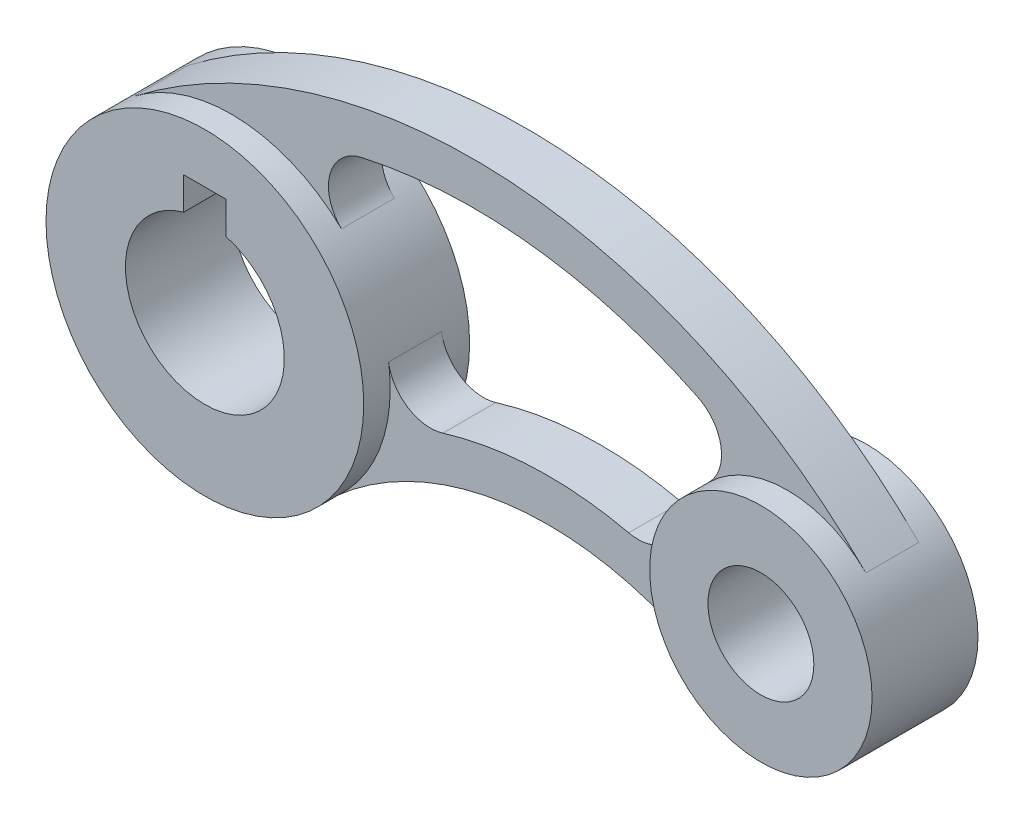
ISO-10303-21;
HEADER;
FILE_DESCRIPTION(('STEP AP214'),'2;1');
FILE_NAME('part.step','',(''),(''),'','','');
FILE_SCHEMA(('AUTOMOTIVE_DESIGN { 1 0 10303 214 1 1 1 1 }'));
ENDSEC;
DATA;
#1=APPLICATION_CONTEXT('core data for automotive mechanical design processes');
#2=APPLICATION_PROTOCOL_DEFINITION('international standard','automotive_design',2000,#1);
#3=PRODUCT_CONTEXT('',#1,'mechanical');
#4=PRODUCT('Part','Part','',(#3));
#5=PRODUCT_RELATED_PRODUCT_CATEGORY('part','',(#4));
#6=PRODUCT_DEFINITION_FORMATION('','',#4);
#7=PRODUCT_DEFINITION_CONTEXT('part definition',#1,'design');
#8=PRODUCT_DEFINITION('design','',#6,#7);
#9=PRODUCT_DEFINITION_SHAPE('','',#8);
#10=(LENGTH_UNIT() NAMED_UNIT(*) SI_UNIT(.MILLI.,.METRE.));
#11=(NAMED_UNIT(*) PLANE_ANGLE_UNIT() SI_UNIT($,.RADIAN.));
#12=(NAMED_UNIT(*) SI_UNIT($,.STERADIAN.) SOLID_ANGLE_UNIT());
#13=UNCERTAINTY_MEASURE_WITH_UNIT(LENGTH_MEASURE(1.E-05),#10,'distance_accuracy_value','');
#14=(GEOMETRIC_REPRESENTATION_CONTEXT(3) GLOBAL_UNCERTAINTY_ASSIGNED_CONTEXT((#13)) GLOBAL_UNIT_ASSIGNED_CONTEXT((#10,
#11,#12)) REPRESENTATION_CONTEXT('',''));
#15=CARTESIAN_POINT('',(0.,0.,0.));
#16=DIRECTION('',(0.,0.,1.));
#17=DIRECTION('',(1.,0.,0.));
#18=AXIS2_PLACEMENT_3D('',#15,#16,#17);
#19=CARTESIAN_POINT('',(-105.,0.,-10.));
#20=DIRECTION('',(0.,0.,1.));
#21=DIRECTION('',(1.,0.,0.));
#22=AXIS2_PLACEMENT_3D('',#19,#20,#21);
#23=CYLINDRICAL_SURFACE('',#22,30.);
#24=CARTESIAN_POINT('',(-105.,0.,-10.));
#25=DIRECTION('',(0.,0.,1.));
#26=DIRECTION('',(1.,0.,0.));
#27=AXIS2_PLACEMENT_3D('',#24,#25,#26);
#28=CIRCLE('',#27,30.);
#29=CARTESIAN_POINT('',(-75.,0.,-10.));
#30=VERTEX_POINT('',#29);
#31=EDGE_CURVE('E287',#30,#30,#28,.T.);
#32=ORIENTED_EDGE('',*,*,#31,.T.);
#33=EDGE_LOOP('',(#32));
#34=FACE_BOUND('',#33,.T.);
#35=CARTESIAN_POINT('',(-105.,0.,10.));
#36=DIRECTION('',(0.,0.,1.));
#37=DIRECTION('',(1.,0.,0.));
#38=AXIS2_PLACEMENT_3D('',#35,#36,#37);
#39=CIRCLE('',#38,30.);
#40=CARTESIAN_POINT('',(-75.,0.,10.));
#41=VERTEX_POINT('',#40);
#42=EDGE_CURVE('E272',#41,#41,#39,.T.);
#43=ORIENTED_EDGE('',*,*,#42,.F.);
#44=EDGE_LOOP('',(#43));
#45=FACE_BOUND('',#44,.T.);
#46=DIRECTION('',(0.,0.,1.));
#47=VECTOR('',#46,1.);
#48=CARTESIAN_POINT('',(-75.3094711139642,4.29796399094698,-5.));
#49=LINE('',#48,#47);
#50=CARTESIAN_POINT('',(-75.3094711139643,4.29796399094698,-5.));
#51=VERTEX_POINT('',#50);
#52=CARTESIAN_POINT('',(-75.3094711139642,4.29796399094699,5.));
#53=VERTEX_POINT('',#52);
#54=EDGE_CURVE('E254',#51,#53,#49,.T.);
#55=ORIENTED_EDGE('',*,*,#54,.F.);
#56=CARTESIAN_POINT('',(-105.,0.,-5.));
#57=DIRECTION('',(0.,0.,1.));
#58=DIRECTION('',(1.,0.,0.));
#59=AXIS2_PLACEMENT_3D('',#56,#57,#58);
#60=CIRCLE('',#59,30.);
#61=CARTESIAN_POINT('',(-85.0571428571429,-22.4116587734954,-5.));
#62=VERTEX_POINT('',#61);
#63=EDGE_CURVE('E245',#62,#51,#60,.T.);
#64=ORIENTED_EDGE('',*,*,#63,.F.);
#65=DIRECTION('',(0.,0.,1.));
#66=VECTOR('',#65,1.);
#67=CARTESIAN_POINT('',(-85.0571428571429,-22.4116587734954,-5.));
#68=LINE('',#67,#66);
#69=CARTESIAN_POINT('',(-85.0571428571429,-22.4116587734954,5.));
#70=VERTEX_POINT('',#69);
#71=EDGE_CURVE('E251',#62,#70,#68,.T.);
#72=ORIENTED_EDGE('',*,*,#71,.T.);
#73=CARTESIAN_POINT('',(-105.,0.,5.));
#74=DIRECTION('',(0.,0.,1.));
#75=DIRECTION('',(1.,0.,0.));
#76=AXIS2_PLACEMENT_3D('',#73,#74,#75);
#77=CIRCLE('',#76,30.);
#78=EDGE_CURVE('E229',#70,#53,#77,.T.);
#79=ORIENTED_EDGE('',*,*,#78,.T.);
#80=EDGE_LOOP('',(#55,#64,#72,#79));
#81=FACE_BOUND('',#80,.T.);
#82=CARTESIAN_POINT('',(-105.,0.,-5.));
#83=DIRECTION('',(0.,0.,1.));
#84=DIRECTION('',(1.,0.,0.));
#85=AXIS2_PLACEMENT_3D('',#82,#83,#84);
#86=CIRCLE('',#85,30.);
#87=CARTESIAN_POINT('',(-84.2069936713874,21.6252372892941,-5.));
#88=VERTEX_POINT('',#87);
#89=CARTESIAN_POINT('',(-123.274285714286,23.7918154337296,-5.));
#90=VERTEX_POINT('',#89);
#91=EDGE_CURVE('E168',#88,#90,#86,.T.);
#92=ORIENTED_EDGE('',*,*,#91,.F.);
#93=DIRECTION('',(0.,0.,-1.));
#94=VECTOR('',#93,1.);
#95=CARTESIAN_POINT('',(-84.2069936713874,21.6252372892941,5.));
#96=LINE('',#95,#94);
#97=CARTESIAN_POINT('',(-84.2069936713874,21.6252372892941,5.));
#98=VERTEX_POINT('',#97);
#99=EDGE_CURVE('E59',#98,#88,#96,.T.);
#100=ORIENTED_EDGE('',*,*,#99,.F.);
#101=CARTESIAN_POINT('',(-105.,0.,5.));
#102=DIRECTION('',(0.,0.,1.));
#103=DIRECTION('',(1.,0.,0.));
#104=AXIS2_PLACEMENT_3D('',#101,#102,#103);
#105=CIRCLE('',#104,30.);
#106=CARTESIAN_POINT('',(-123.274285714286,23.7918154337296,5.));
#107=VERTEX_POINT('',#106);
#108=EDGE_CURVE('E186',#98,#107,#105,.T.);
#109=ORIENTED_EDGE('',*,*,#108,.T.);
#110=DIRECTION('',(0.,0.,-1.));
#111=VECTOR('',#110,1.);
#112=CARTESIAN_POINT('',(-123.274285714286,23.7918154337296,5.));
#113=LINE('',#112,#111);
#114=EDGE_CURVE('E62',#107,#90,#113,.T.);
#115=ORIENTED_EDGE('',*,*,#114,.T.);
#116=EDGE_LOOP('',(#92,#100,#109,#115));
#117=FACE_BOUND('',#116,.T.);
#118=ADVANCED_FACE('F41',(#34,#45,#81,#117),#23,.T.);
#119=CARTESIAN_POINT('',(-105.,0.,-10.));
#120=DIRECTION('',(0.,0.,1.));
#121=DIRECTION('',(1.,0.,0.));
#122=AXIS2_PLACEMENT_3D('',#119,#120,#121);
#123=CYLINDRICAL_SURFACE('',#122,15.);
#124=DIRECTION('',(0.,0.,1.));
#125=VECTOR('',#124,1.);
#126=CARTESIAN_POINT('',(-109.,14.4568322948009,-10.));
#127=LINE('',#126,#125);
#128=CARTESIAN_POINT('',(-109.,14.4568322948009,-10.));
#129=VERTEX_POINT('',#128);
#130=CARTESIAN_POINT('',(-109.,14.4568322948009,10.));
#131=VERTEX_POINT('',#130);
#132=EDGE_CURVE('E44',#129,#131,#127,.T.);
#133=ORIENTED_EDGE('',*,*,#132,.T.);
#134=CARTESIAN_POINT('',(-105.,0.,10.));
#135=DIRECTION('',(0.,0.,1.));
#136=DIRECTION('',(1.,0.,0.));
#137=AXIS2_PLACEMENT_3D('',#134,#135,#136);
#138=CIRCLE('',#137,15.);
#139=CARTESIAN_POINT('',(-101.,14.4568322948009,10.));
#140=VERTEX_POINT('',#139);
#141=EDGE_CURVE('E252',#131,#140,#138,.T.);
#142=ORIENTED_EDGE('',*,*,#141,.T.);
#143=DIRECTION('',(0.,0.,1.));
#144=VECTOR('',#143,1.);
#145=CARTESIAN_POINT('',(-101.,14.4568322948009,-10.));
#146=LINE('',#145,#144);
#147=CARTESIAN_POINT('',(-101.,14.4568322948009,-10.));
#148=VERTEX_POINT('',#147);
#149=EDGE_CURVE('E11',#148,#140,#146,.T.);
#150=ORIENTED_EDGE('',*,*,#149,.F.);
#151=CARTESIAN_POINT('',(-105.,0.,-10.));
#152=DIRECTION('',(0.,0.,1.));
#153=DIRECTION('',(1.,0.,0.));
#154=AXIS2_PLACEMENT_3D('',#151,#152,#153);
#155=CIRCLE('',#154,15.);
#156=EDGE_CURVE('E277',#129,#148,#155,.T.);
#157=ORIENTED_EDGE('',*,*,#156,.F.);
#158=EDGE_LOOP('',(#133,#142,#150,#157));
#159=FACE_BOUND('',#158,.T.);
#160=ADVANCED_FACE('F43',(#159),#123,.F.);
#161=CARTESIAN_POINT('',(-101.,0.,-10.));
#162=DIRECTION('',(-1.,0.,0.));
#163=DIRECTION('',(0.,0.,1.));
#164=AXIS2_PLACEMENT_3D('',#161,#162,#163);
#165=PLANE('',#164);
#166=ORIENTED_EDGE('',*,*,#149,.T.);
#167=DIRECTION('',(0.,-1.,0.));
#168=VECTOR('',#167,1.);
#169=CARTESIAN_POINT('',(-101.,0.,10.));
#170=LINE('',#169,#168);
#171=CARTESIAN_POINT('',(-101.,20.5784582370718,10.));
#172=VERTEX_POINT('',#171);
#173=EDGE_CURVE('E269',#172,#140,#170,.T.);
#174=ORIENTED_EDGE('',*,*,#173,.F.);
#175=DIRECTION('',(0.,0.,1.));
#176=VECTOR('',#175,1.);
#177=CARTESIAN_POINT('',(-101.,20.5784582370718,-10.));
#178=LINE('',#177,#176);
#179=CARTESIAN_POINT('',(-101.,20.5784582370718,-10.));
#180=VERTEX_POINT('',#179);
#181=EDGE_CURVE('E49',#180,#172,#178,.T.);
#182=ORIENTED_EDGE('',*,*,#181,.F.);
#183=DIRECTION('',(0.,-1.,0.));
#184=VECTOR('',#183,1.);
#185=CARTESIAN_POINT('',(-101.,0.,-10.));
#186=LINE('',#185,#184);
#187=EDGE_CURVE('E285',#180,#148,#186,.T.);
#188=ORIENTED_EDGE('',*,*,#187,.T.);
#189=EDGE_LOOP('',(#166,#174,#182,#188));
#190=FACE_BOUND('',#189,.T.);
#191=ADVANCED_FACE('F311',(#190),#165,.T.);
#192=CARTESIAN_POINT('',(0.,20.5784582370718,-10.));
#193=DIRECTION('',(0.,-1.,0.));
#194=DIRECTION('',(0.,0.,-1.));
#195=AXIS2_PLACEMENT_3D('',#192,#193,#194);
#196=PLANE('',#195);
#197=ORIENTED_EDGE('',*,*,#181,.T.);
#198=DIRECTION('',(1.,0.,0.));
#199=VECTOR('',#198,1.);
#200=CARTESIAN_POINT('',(0.,20.5784582370718,10.));
#201=LINE('',#200,#199);
#202=CARTESIAN_POINT('',(-109.,20.5784582370718,10.));
#203=VERTEX_POINT('',#202);
#204=EDGE_CURVE('E270',#203,#172,#201,.T.);
#205=ORIENTED_EDGE('',*,*,#204,.F.);
#206=DIRECTION('',(0.,0.,1.));
#207=VECTOR('',#206,1.);
#208=CARTESIAN_POINT('',(-109.,20.5784582370718,-10.));
#209=LINE('',#208,#207);
#210=CARTESIAN_POINT('',(-109.,20.5784582370718,-10.));
#211=VERTEX_POINT('',#210);
#212=EDGE_CURVE('E286',#211,#203,#209,.T.);
#213=ORIENTED_EDGE('',*,*,#212,.F.);
#214=DIRECTION('',(1.,0.,0.));
#215=VECTOR('',#214,1.);
#216=CARTESIAN_POINT('',(0.,20.5784582370718,-10.));
#217=LINE('',#216,#215);
#218=EDGE_CURVE('E278',#211,#180,#217,.T.);
#219=ORIENTED_EDGE('',*,*,#218,.T.);
#220=EDGE_LOOP('',(#197,#205,#213,#219));
#221=FACE_BOUND('',#220,.T.);
#222=ADVANCED_FACE('F308',(#221),#196,.T.);
#223=CARTESIAN_POINT('',(-109.,0.,-10.));
#224=DIRECTION('',(-1.,0.,0.));
#225=DIRECTION('',(0.,0.,1.));
#226=AXIS2_PLACEMENT_3D('',#223,#224,#225);
#227=PLANE('',#226);
#228=ORIENTED_EDGE('',*,*,#212,.T.);
#229=DIRECTION('',(0.,-1.,0.));
#230=VECTOR('',#229,1.);
#231=CARTESIAN_POINT('',(-109.,0.,10.));
#232=LINE('',#231,#230);
#233=EDGE_CURVE('E262',#203,#131,#232,.T.);
#234=ORIENTED_EDGE('',*,*,#233,.T.);
#235=ORIENTED_EDGE('',*,*,#132,.F.);
#236=DIRECTION('',(0.,-1.,0.));
#237=VECTOR('',#236,1.);
#238=CARTESIAN_POINT('',(-109.,0.,-10.));
#239=LINE('',#238,#237);
#240=EDGE_CURVE('E279',#211,#129,#239,.T.);
#241=ORIENTED_EDGE('',*,*,#240,.F.);
#242=EDGE_LOOP('',(#228,#234,#235,#241));
#243=FACE_BOUND('',#242,.T.);
#244=ADVANCED_FACE('F304',(#243),#227,.F.);
#245=CARTESIAN_POINT('',(0.,0.,-10.));
#246=DIRECTION('',(0.,0.,1.));
#247=DIRECTION('',(1.,0.,0.));
#248=AXIS2_PLACEMENT_3D('',#245,#246,#247);
#249=PLANE('',#248);
#250=ORIENTED_EDGE('',*,*,#156,.T.);
#251=ORIENTED_EDGE('',*,*,#187,.F.);
#252=ORIENTED_EDGE('',*,*,#218,.F.);
#253=ORIENTED_EDGE('',*,*,#240,.T.);
#254=EDGE_LOOP('',(#250,#251,#252,#253));
#255=FACE_BOUND('',#254,.T.);
#256=ORIENTED_EDGE('',*,*,#31,.F.);
#257=EDGE_LOOP('',(#256));
#258=FACE_BOUND('',#257,.T.);
#259=ADVANCED_FACE('F303',(#255,#258),#249,.F.);
#260=CARTESIAN_POINT('',(0.,0.,10.));
#261=DIRECTION('',(0.,0.,1.));
#262=DIRECTION('',(1.,0.,0.));
#263=AXIS2_PLACEMENT_3D('',#260,#261,#262);
#264=PLANE('',#263);
#265=ORIENTED_EDGE('',*,*,#141,.F.);
#266=ORIENTED_EDGE('',*,*,#233,.F.);
#267=ORIENTED_EDGE('',*,*,#204,.T.);
#268=ORIENTED_EDGE('',*,*,#173,.T.);
#269=EDGE_LOOP('',(#265,#266,#267,#268));
#270=FACE_BOUND('',#269,.T.);
#271=ORIENTED_EDGE('',*,*,#42,.T.);
#272=EDGE_LOOP('',(#271));
#273=FACE_BOUND('',#272,.T.);
#274=ADVANCED_FACE('F297',(#270,#273),#264,.T.);
#275=CARTESIAN_POINT('',(-45.1714285714286,-67.2349763204861,-5.));
#276=DIRECTION('',(0.,0.,1.));
#277=DIRECTION('',(1.,0.,0.));
#278=AXIS2_PLACEMENT_3D('',#275,#276,#277);
#279=CYLINDRICAL_SURFACE('',#278,60.);
#280=CARTESIAN_POINT('',(-45.1714285714286,-67.2349763204861,5.));
#281=DIRECTION('',(0.,0.,1.));
#282=DIRECTION('',(1.,0.,0.));
#283=AXIS2_PLACEMENT_3D('',#280,#281,#282);
#284=CIRCLE('',#283,60.);
#285=CARTESIAN_POINT('',(-11.7111111111111,-17.4312901571631,5.));
#286=VERTEX_POINT('',#285);
#287=EDGE_CURVE('E228',#286,#70,#284,.T.);
#288=ORIENTED_EDGE('',*,*,#287,.T.);
#289=ORIENTED_EDGE('',*,*,#71,.F.);
#290=CARTESIAN_POINT('',(-45.1714285714286,-67.2349763204861,-5.));
#291=DIRECTION('',(0.,0.,1.));
#292=DIRECTION('',(1.,0.,0.));
#293=AXIS2_PLACEMENT_3D('',#290,#291,#292);
#294=CIRCLE('',#293,60.);
#295=CARTESIAN_POINT('',(-11.7111111111111,-17.4312901571631,-5.));
#296=VERTEX_POINT('',#295);
#297=EDGE_CURVE('E247',#296,#62,#294,.T.);
#298=ORIENTED_EDGE('',*,*,#297,.F.);
#299=DIRECTION('',(0.,0.,1.));
#300=VECTOR('',#299,1.);
#301=CARTESIAN_POINT('',(-11.7111111111111,-17.4312901571631,-5.));
#302=LINE('',#301,#300);
#303=EDGE_CURVE('E248',#296,#286,#302,.T.);
#304=ORIENTED_EDGE('',*,*,#303,.T.);
#305=EDGE_LOOP('',(#288,#289,#298,#304));
#306=FACE_BOUND('',#305,.T.);
#307=ADVANCED_FACE('F363',(#306),#279,.F.);
#308=CARTESIAN_POINT('',(-67.3919967443547,5.44408772186619,-5.));
#309=DIRECTION('',(0.,0.,1.));
#310=DIRECTION('',(1.,0.,0.));
#311=AXIS2_PLACEMENT_3D('',#308,#309,#310);
#312=CYLINDRICAL_SURFACE('',#311,8.);
#313=CARTESIAN_POINT('',(-67.3919967443547,5.44408772186619,5.));
#314=DIRECTION('',(0.,0.,1.));
#315=DIRECTION('',(1.,0.,0.));
#316=AXIS2_PLACEMENT_3D('',#313,#314,#315);
#317=CIRCLE('',#316,8.);
#318=CARTESIAN_POINT('',(-65.0529895682572,-2.20634007206563,5.));
#319=VERTEX_POINT('',#318);
#320=EDGE_CURVE('E224',#53,#319,#317,.T.);
#321=ORIENTED_EDGE('',*,*,#320,.T.);
#322=DIRECTION('',(0.,0.,1.));
#323=VECTOR('',#322,1.);
#324=CARTESIAN_POINT('',(-65.0529895682572,-2.20634007206563,-5.));
#325=LINE('',#324,#323);
#326=CARTESIAN_POINT('',(-65.0529895682572,-2.20634007206563,-5.));
#327=VERTEX_POINT('',#326);
#328=EDGE_CURVE('E260',#327,#319,#325,.T.);
#329=ORIENTED_EDGE('',*,*,#328,.F.);
#330=CARTESIAN_POINT('',(-67.3919967443547,5.44408772186619,-5.));
#331=DIRECTION('',(0.,0.,1.));
#332=DIRECTION('',(1.,0.,0.));
#333=AXIS2_PLACEMENT_3D('',#330,#331,#332);
#334=CIRCLE('',#333,8.);
#335=EDGE_CURVE('E244',#51,#327,#334,.T.);
#336=ORIENTED_EDGE('',*,*,#335,.F.);
#337=ORIENTED_EDGE('',*,*,#54,.T.);
#338=EDGE_LOOP('',(#321,#329,#336,#337));
#339=FACE_BOUND('',#338,.T.);
#340=ADVANCED_FACE('F504',(#339),#312,.F.);
#341=CARTESIAN_POINT('',(-45.1714285714286,-67.2349763204861,-5.));
#342=DIRECTION('',(0.,0.,1.));
#343=DIRECTION('',(1.,0.,0.));
#344=AXIS2_PLACEMENT_3D('',#341,#342,#343);
#345=CYLINDRICAL_SURFACE('',#344,68.);
#346=CARTESIAN_POINT('',(-45.1714285714286,-67.2349763204861,5.));
#347=DIRECTION('',(0.,0.,1.));
#348=DIRECTION('',(1.,0.,0.));
#349=AXIS2_PLACEMENT_3D('',#346,#347,#348);
#350=CIRCLE('',#349,68.);
#351=CARTESIAN_POINT('',(-29.9698424769779,-0.955931515864719,5.));
#352=VERTEX_POINT('',#351);
#353=EDGE_CURVE('E219',#352,#319,#350,.T.);
#354=ORIENTED_EDGE('',*,*,#353,.F.);
#355=DIRECTION('',(0.,0.,1.));
#356=VECTOR('',#355,1.);
#357=CARTESIAN_POINT('',(-29.9698424769779,-0.955931515864719,-5.));
#358=LINE('',#357,#356);
#359=CARTESIAN_POINT('',(-29.9698424769779,-0.955931515864719,-5.));
#360=VERTEX_POINT('',#359);
#361=EDGE_CURVE('E259',#360,#352,#358,.T.);
#362=ORIENTED_EDGE('',*,*,#361,.F.);
#363=CARTESIAN_POINT('',(-45.1714285714286,-67.2349763204861,-5.));
#364=DIRECTION('',(0.,0.,1.));
#365=DIRECTION('',(1.,0.,0.));
#366=AXIS2_PLACEMENT_3D('',#363,#364,#365);
#367=CIRCLE('',#366,68.);
#368=EDGE_CURVE('E236',#360,#327,#367,.T.);
#369=ORIENTED_EDGE('',*,*,#368,.T.);
#370=ORIENTED_EDGE('',*,*,#328,.T.);
#371=EDGE_LOOP('',(#354,#362,#369,#370));
#372=FACE_BOUND('',#371,.T.);
#373=ADVANCED_FACE('F495',(#372),#345,.T.);
#374=CARTESIAN_POINT('',(-28.1814205835132,6.84160316703191,-5.));
#375=DIRECTION('',(0.,0.,1.));
#376=DIRECTION('',(1.,0.,0.));
#377=AXIS2_PLACEMENT_3D('',#374,#375,#376);
#378=CYLINDRICAL_SURFACE('',#377,8.);
#379=CARTESIAN_POINT('',(-28.1814205835132,6.84160316703191,5.));
#380=DIRECTION('',(0.,0.,1.));
#381=DIRECTION('',(1.,0.,0.));
#382=AXIS2_PLACEMENT_3D('',#379,#380,#381);
#383=CIRCLE('',#382,8.);
#384=CARTESIAN_POINT('',(-20.4072355949578,4.95426436233345,5.));
#385=VERTEX_POINT('',#384);
#386=EDGE_CURVE('E220',#385,#352,#383,.F.);
#387=ORIENTED_EDGE('',*,*,#386,.F.);
#388=DIRECTION('',(0.,0.,1.));
#389=VECTOR('',#388,1.);
#390=CARTESIAN_POINT('',(-20.4072355949578,4.95426436233345,-5.));
#391=LINE('',#390,#389);
#392=CARTESIAN_POINT('',(-20.4072355949578,4.95426436233345,-5.));
#393=VERTEX_POINT('',#392);
#394=EDGE_CURVE('E246',#393,#385,#391,.T.);
#395=ORIENTED_EDGE('',*,*,#394,.F.);
#396=CARTESIAN_POINT('',(-28.1814205835132,6.84160316703191,-5.));
#397=DIRECTION('',(0.,0.,1.));
#398=DIRECTION('',(1.,0.,0.));
#399=AXIS2_PLACEMENT_3D('',#396,#397,#398);
#400=CIRCLE('',#399,8.);
#401=EDGE_CURVE('E233',#393,#360,#400,.F.);
#402=ORIENTED_EDGE('',*,*,#401,.T.);
#403=ORIENTED_EDGE('',*,*,#361,.T.);
#404=EDGE_LOOP('',(#387,#395,#402,#403));
#405=FACE_BOUND('',#404,.T.);
#406=ADVANCED_FACE('F483',(#405),#378,.F.);
#407=CARTESIAN_POINT('',(0.,0.,-5.));
#408=DIRECTION('',(0.,0.,1.));
#409=DIRECTION('',(1.,0.,0.));
#410=AXIS2_PLACEMENT_3D('',#407,#408,#409);
#411=PLANE('',#410);
#412=CARTESIAN_POINT('',(0.,0.,-5.));
#413=DIRECTION('',(0.,0.,1.));
#414=DIRECTION('',(1.,0.,0.));
#415=AXIS2_PLACEMENT_3D('',#412,#413,#414);
#416=CIRCLE('',#415,21.);
#417=EDGE_CURVE('E235',#393,#296,#416,.T.);
#418=ORIENTED_EDGE('',*,*,#417,.T.);
#419=ORIENTED_EDGE('',*,*,#297,.T.);
#420=ORIENTED_EDGE('',*,*,#63,.T.);
#421=ORIENTED_EDGE('',*,*,#335,.T.);
#422=ORIENTED_EDGE('',*,*,#368,.F.);
#423=ORIENTED_EDGE('',*,*,#401,.F.);
#424=EDGE_LOOP('',(#418,#419,#420,#421,#422,#423));
#425=FACE_BOUND('',#424,.T.);
#426=ADVANCED_FACE('F474',(#425),#411,.F.);
#427=CARTESIAN_POINT('',(0.,0.,5.));
#428=DIRECTION('',(0.,0.,1.));
#429=DIRECTION('',(1.,0.,0.));
#430=AXIS2_PLACEMENT_3D('',#427,#428,#429);
#431=PLANE('',#430);
#432=CARTESIAN_POINT('',(0.,0.,5.));
#433=DIRECTION('',(0.,0.,1.));
#434=DIRECTION('',(1.,0.,0.));
#435=AXIS2_PLACEMENT_3D('',#432,#433,#434);
#436=CIRCLE('',#435,21.);
#437=EDGE_CURVE('E212',#385,#286,#436,.T.);
#438=ORIENTED_EDGE('',*,*,#437,.F.);
#439=ORIENTED_EDGE('',*,*,#386,.T.);
#440=ORIENTED_EDGE('',*,*,#353,.T.);
#441=ORIENTED_EDGE('',*,*,#320,.F.);
#442=ORIENTED_EDGE('',*,*,#78,.F.);
#443=ORIENTED_EDGE('',*,*,#287,.F.);
#444=EDGE_LOOP('',(#438,#439,#440,#441,#442,#443));
#445=FACE_BOUND('',#444,.T.);
#446=ADVANCED_FACE('F371',(#445),#431,.T.);
#447=CARTESIAN_POINT('',(0.,0.,-10.));
#448=DIRECTION('',(0.,0.,1.));
#449=DIRECTION('',(1.,0.,0.));
#450=AXIS2_PLACEMENT_3D('',#447,#448,#449);
#451=CYLINDRICAL_SURFACE('',#450,21.);
#452=DIRECTION('',(0.,0.,-1.));
#453=VECTOR('',#452,1.);
#454=CARTESIAN_POINT('',(-14.7966570747391,14.9016421716727,5.));
#455=LINE('',#454,#453);
#456=CARTESIAN_POINT('',(-14.7966570747391,14.9016421716727,5.));
#457=VERTEX_POINT('',#456);
#458=CARTESIAN_POINT('',(-14.7966570747391,14.9016421716727,-5.));
#459=VERTEX_POINT('',#458);
#460=EDGE_CURVE('E193',#457,#459,#455,.T.);
#461=ORIENTED_EDGE('',*,*,#460,.T.);
#462=CARTESIAN_POINT('',(0.,0.,-5.));
#463=DIRECTION('',(0.,0.,1.));
#464=DIRECTION('',(1.,0.,0.));
#465=AXIS2_PLACEMENT_3D('',#462,#463,#464);
#466=CIRCLE('',#465,21.);
#467=CARTESIAN_POINT('',(14.8285714285714,14.869884646081,-5.));
#468=VERTEX_POINT('',#467);
#469=EDGE_CURVE('E562',#468,#459,#466,.T.);
#470=ORIENTED_EDGE('',*,*,#469,.F.);
#471=DIRECTION('',(0.,0.,-1.));
#472=VECTOR('',#471,1.);
#473=CARTESIAN_POINT('',(14.8285714285714,14.869884646081,5.));
#474=LINE('',#473,#472);
#475=CARTESIAN_POINT('',(14.8285714285714,14.869884646081,5.));
#476=VERTEX_POINT('',#475);
#477=EDGE_CURVE('E199',#476,#468,#474,.T.);
#478=ORIENTED_EDGE('',*,*,#477,.F.);
#479=CARTESIAN_POINT('',(0.,0.,5.));
#480=DIRECTION('',(0.,0.,1.));
#481=DIRECTION('',(1.,0.,0.));
#482=AXIS2_PLACEMENT_3D('',#479,#480,#481);
#483=CIRCLE('',#482,21.);
#484=EDGE_CURVE('E179',#476,#457,#483,.T.);
#485=ORIENTED_EDGE('',*,*,#484,.T.);
#486=EDGE_LOOP('',(#461,#470,#478,#485));
#487=FACE_BOUND('',#486,.T.);
#488=CARTESIAN_POINT('',(0.,0.,10.));
#489=DIRECTION('',(0.,0.,1.));
#490=DIRECTION('',(1.,0.,0.));
#491=AXIS2_PLACEMENT_3D('',#488,#489,#490);
#492=CIRCLE('',#491,21.);
#493=CARTESIAN_POINT('',(21.,0.,10.));
#494=VERTEX_POINT('',#493);
#495=EDGE_CURVE('E202',#494,#494,#492,.T.);
#496=ORIENTED_EDGE('',*,*,#495,.F.);
#497=EDGE_LOOP('',(#496));
#498=FACE_BOUND('',#497,.T.);
#499=CARTESIAN_POINT('',(0.,0.,-10.));
#500=DIRECTION('',(0.,0.,1.));
#501=DIRECTION('',(1.,0.,0.));
#502=AXIS2_PLACEMENT_3D('',#499,#500,#501);
#503=CIRCLE('',#502,21.);
#504=CARTESIAN_POINT('',(21.,0.,-10.));
#505=VERTEX_POINT('',#504);
#506=EDGE_CURVE('E211',#505,#505,#503,.T.);
#507=ORIENTED_EDGE('',*,*,#506,.T.);
#508=EDGE_LOOP('',(#507));
#509=FACE_BOUND('',#508,.T.);
#510=ORIENTED_EDGE('',*,*,#417,.F.);
#511=ORIENTED_EDGE('',*,*,#394,.T.);
#512=ORIENTED_EDGE('',*,*,#437,.T.);
#513=ORIENTED_EDGE('',*,*,#303,.F.);
#514=EDGE_LOOP('',(#510,#511,#512,#513));
#515=FACE_BOUND('',#514,.T.);
#516=ADVANCED_FACE('F364',(#487,#498,#509,#515),#451,.T.);
#517=CARTESIAN_POINT('',(0.,0.,-10.));
#518=DIRECTION('',(0.,0.,1.));
#519=DIRECTION('',(1.,0.,0.));
#520=AXIS2_PLACEMENT_3D('',#517,#518,#519);
#521=CYLINDRICAL_SURFACE('',#520,10.);
#522=CARTESIAN_POINT('',(0.,0.,-10.));
#523=DIRECTION('',(0.,0.,1.));
#524=DIRECTION('',(1.,0.,0.));
#525=AXIS2_PLACEMENT_3D('',#522,#523,#524);
#526=CIRCLE('',#525,10.);
#527=CARTESIAN_POINT('',(10.,0.,-10.));
#528=VERTEX_POINT('',#527);
#529=EDGE_CURVE('E208',#528,#528,#526,.T.);
#530=ORIENTED_EDGE('',*,*,#529,.F.);
#531=EDGE_LOOP('',(#530));
#532=FACE_BOUND('',#531,.T.);
#533=CARTESIAN_POINT('',(0.,0.,10.));
#534=DIRECTION('',(0.,0.,1.));
#535=DIRECTION('',(1.,0.,0.));
#536=AXIS2_PLACEMENT_3D('',#533,#534,#535);
#537=CIRCLE('',#536,10.);
#538=CARTESIAN_POINT('',(10.,0.,10.));
#539=VERTEX_POINT('',#538);
#540=EDGE_CURVE('E205',#539,#539,#537,.T.);
#541=ORIENTED_EDGE('',*,*,#540,.T.);
#542=EDGE_LOOP('',(#541));
#543=FACE_BOUND('',#542,.T.);
#544=ADVANCED_FACE('F367',(#532,#543),#521,.F.);
#545=CARTESIAN_POINT('',(0.,0.,-10.));
#546=DIRECTION('',(0.,0.,1.));
#547=DIRECTION('',(1.,0.,0.));
#548=AXIS2_PLACEMENT_3D('',#545,#546,#547);
#549=PLANE('',#548);
#550=ORIENTED_EDGE('',*,*,#529,.T.);
#551=EDGE_LOOP('',(#550));
#552=FACE_BOUND('',#551,.T.);
#553=ORIENTED_EDGE('',*,*,#506,.F.);
#554=EDGE_LOOP('',(#553));
#555=FACE_BOUND('',#554,.T.);
#556=ADVANCED_FACE('F387',(#552,#555),#549,.F.);
#557=CARTESIAN_POINT('',(0.,0.,10.));
#558=DIRECTION('',(0.,0.,1.));
#559=DIRECTION('',(1.,0.,0.));
#560=AXIS2_PLACEMENT_3D('',#557,#558,#559);
#561=PLANE('',#560);
#562=ORIENTED_EDGE('',*,*,#540,.F.);
#563=EDGE_LOOP('',(#562));
#564=FACE_BOUND('',#563,.T.);
#565=ORIENTED_EDGE('',*,*,#495,.T.);
#566=EDGE_LOOP('',(#565));
#567=FACE_BOUND('',#566,.T.);
#568=ADVANCED_FACE('F393',(#564,#567),#561,.T.);
#569=CARTESIAN_POINT('',(-59.3142857142857,-59.4795385843239,5.));
#570=DIRECTION('',(0.,0.,-1.));
#571=DIRECTION('',(-1.,0.,0.));
#572=AXIS2_PLACEMENT_3D('',#569,#570,#571);
#573=CYLINDRICAL_SURFACE('',#572,105.);
#574=ORIENTED_EDGE('',*,*,#477,.T.);
#575=CARTESIAN_POINT('',(-59.3142857142857,-59.4795385843239,-5.));
#576=DIRECTION('',(0.,0.,1.));
#577=DIRECTION('',(1.,0.,0.));
#578=AXIS2_PLACEMENT_3D('',#575,#576,#577);
#579=CIRCLE('',#578,105.);
#580=EDGE_CURVE('E557',#90,#468,#579,.F.);
#581=ORIENTED_EDGE('',*,*,#580,.F.);
#582=ORIENTED_EDGE('',*,*,#114,.F.);
#583=CARTESIAN_POINT('',(-59.3142857142857,-59.4795385843239,5.));
#584=DIRECTION('',(0.,0.,1.));
#585=DIRECTION('',(1.,0.,0.));
#586=AXIS2_PLACEMENT_3D('',#583,#584,#585);
#587=CIRCLE('',#586,105.);
#588=EDGE_CURVE('E184',#107,#476,#587,.F.);
#589=ORIENTED_EDGE('',*,*,#588,.T.);
#590=EDGE_LOOP('',(#574,#581,#582,#589));
#591=FACE_BOUND('',#590,.T.);
#592=ADVANCED_FACE('F405',(#591),#573,.T.);
#593=CARTESIAN_POINT('',(-78.6621919837574,27.3919672331059,5.));
#594=DIRECTION('',(0.,0.,-1.));
#595=DIRECTION('',(-1.,0.,0.));
#596=AXIS2_PLACEMENT_3D('',#593,#594,#595);
#597=CYLINDRICAL_SURFACE('',#596,8.);
#598=ORIENTED_EDGE('',*,*,#99,.T.);
#599=CARTESIAN_POINT('',(-78.6621919837574,27.3919672331059,-5.));
#600=DIRECTION('',(0.,0.,1.));
#601=DIRECTION('',(1.,0.,0.));
#602=AXIS2_PLACEMENT_3D('',#599,#600,#601);
#603=CIRCLE('',#602,8.);
#604=CARTESIAN_POINT('',(-80.4013296259571,35.2006419133243,-5.));
#605=VERTEX_POINT('',#604);
#606=EDGE_CURVE('E170',#605,#88,#603,.T.);
#607=ORIENTED_EDGE('',*,*,#606,.F.);
#608=DIRECTION('',(0.,0.,-1.));
#609=VECTOR('',#608,1.);
#610=CARTESIAN_POINT('',(-80.4013296259571,35.2006419133243,5.));
#611=LINE('',#610,#609);
#612=CARTESIAN_POINT('',(-80.4013296259571,35.2006419133243,5.));
#613=VERTEX_POINT('',#612);
#614=EDGE_CURVE('E160',#613,#605,#611,.T.);
#615=ORIENTED_EDGE('',*,*,#614,.F.);
#616=CARTESIAN_POINT('',(-78.6621919837574,27.3919672331059,5.));
#617=DIRECTION('',(0.,0.,1.));
#618=DIRECTION('',(1.,0.,0.));
#619=AXIS2_PLACEMENT_3D('',#616,#617,#618);
#620=CIRCLE('',#619,8.);
#621=EDGE_CURVE('E188',#613,#98,#620,.T.);
#622=ORIENTED_EDGE('',*,*,#621,.T.);
#623=EDGE_LOOP('',(#598,#607,#615,#622));
#624=FACE_BOUND('',#623,.T.);
#625=ADVANCED_FACE('F169',(#624),#597,.F.);
#626=CARTESIAN_POINT('',(-59.3142857142857,-59.4795385843239,5.));
#627=DIRECTION('',(0.,0.,-1.));
#628=DIRECTION('',(-1.,0.,0.));
#629=AXIS2_PLACEMENT_3D('',#626,#627,#628);
#630=CYLINDRICAL_SURFACE('',#629,97.);
#631=ORIENTED_EDGE('',*,*,#614,.T.);
#632=CARTESIAN_POINT('',(-59.3142857142857,-59.4795385843239,-5.));
#633=DIRECTION('',(0.,0.,1.));
#634=DIRECTION('',(1.,0.,0.));
#635=AXIS2_PLACEMENT_3D('',#632,#633,#634);
#636=CIRCLE('',#635,97.);
#637=CARTESIAN_POINT('',(-16.9385748267742,27.7746826704557,-5.));
#638=VERTEX_POINT('',#637);
#639=EDGE_CURVE('E161',#605,#638,#636,.F.);
#640=ORIENTED_EDGE('',*,*,#639,.T.);
#641=DIRECTION('',(0.,0.,-1.));
#642=VECTOR('',#641,1.);
#643=CARTESIAN_POINT('',(-16.9385748267742,27.7746826704557,5.));
#644=LINE('',#643,#642);
#645=CARTESIAN_POINT('',(-16.9385748267742,27.7746826704557,5.));
#646=VERTEX_POINT('',#645);
#647=EDGE_CURVE('E163',#646,#638,#644,.T.);
#648=ORIENTED_EDGE('',*,*,#647,.F.);
#649=CARTESIAN_POINT('',(-59.3142857142857,-59.4795385843239,5.));
#650=DIRECTION('',(0.,0.,1.));
#651=DIRECTION('',(1.,0.,0.));
#652=AXIS2_PLACEMENT_3D('',#649,#650,#651);
#653=CIRCLE('',#652,97.);
#654=EDGE_CURVE('E165',#613,#646,#653,.F.);
#655=ORIENTED_EDGE('',*,*,#654,.F.);
#656=EDGE_LOOP('',(#631,#640,#648,#655));
#657=FACE_BOUND('',#656,.T.);
#658=ADVANCED_FACE('F158',(#657),#630,.F.);
#659=CARTESIAN_POINT('',(-20.4334788174968,20.5784582370718,5.));
#660=DIRECTION('',(0.,0.,-1.));
#661=DIRECTION('',(-1.,0.,0.));
#662=AXIS2_PLACEMENT_3D('',#659,#660,#661);
#663=CYLINDRICAL_SURFACE('',#662,8.);
#664=ORIENTED_EDGE('',*,*,#647,.T.);
#665=CARTESIAN_POINT('',(-20.4334788174968,20.5784582370718,-5.));
#666=DIRECTION('',(0.,0.,1.));
#667=DIRECTION('',(1.,0.,0.));
#668=AXIS2_PLACEMENT_3D('',#665,#666,#667);
#669=CIRCLE('',#668,8.);
#670=EDGE_CURVE('E177',#459,#638,#669,.T.);
#671=ORIENTED_EDGE('',*,*,#670,.F.);
#672=ORIENTED_EDGE('',*,*,#460,.F.);
#673=CARTESIAN_POINT('',(-20.4334788174968,20.5784582370718,5.));
#674=DIRECTION('',(0.,0.,1.));
#675=DIRECTION('',(1.,0.,0.));
#676=AXIS2_PLACEMENT_3D('',#673,#674,#675);
#677=CIRCLE('',#676,8.);
#678=EDGE_CURVE('E195',#457,#646,#677,.T.);
#679=ORIENTED_EDGE('',*,*,#678,.T.);
#680=EDGE_LOOP('',(#664,#671,#672,#679));
#681=FACE_BOUND('',#680,.T.);
#682=ADVANCED_FACE('F430',(#681),#663,.F.);
#683=CARTESIAN_POINT('',(0.,0.,5.));
#684=DIRECTION('',(0.,0.,1.));
#685=DIRECTION('',(1.,0.,0.));
#686=AXIS2_PLACEMENT_3D('',#683,#684,#685);
#687=PLANE('',#686);
#688=ORIENTED_EDGE('',*,*,#484,.F.);
#689=ORIENTED_EDGE('',*,*,#588,.F.);
#690=ORIENTED_EDGE('',*,*,#108,.F.);
#691=ORIENTED_EDGE('',*,*,#621,.F.);
#692=ORIENTED_EDGE('',*,*,#654,.T.);
#693=ORIENTED_EDGE('',*,*,#678,.F.);
#694=EDGE_LOOP('',(#688,#689,#690,#691,#692,#693));
#695=FACE_BOUND('',#694,.T.);
#696=ADVANCED_FACE('F434',(#695),#687,.T.);
#697=CARTESIAN_POINT('',(0.,0.,-5.));
#698=DIRECTION('',(0.,0.,1.));
#699=DIRECTION('',(1.,0.,0.));
#700=AXIS2_PLACEMENT_3D('',#697,#698,#699);
#701=PLANE('',#700);
#702=ORIENTED_EDGE('',*,*,#469,.T.);
#703=ORIENTED_EDGE('',*,*,#670,.T.);
#704=ORIENTED_EDGE('',*,*,#639,.F.);
#705=ORIENTED_EDGE('',*,*,#606,.T.);
#706=ORIENTED_EDGE('',*,*,#91,.T.);
#707=ORIENTED_EDGE('',*,*,#580,.T.);
#708=EDGE_LOOP('',(#702,#703,#704,#705,#706,#707));
#709=FACE_BOUND('',#708,.T.);
#710=ADVANCED_FACE('F173',(#709),#701,.F.);
#711=CLOSED_SHELL('',(#118,#160,#191,#222,#244,#259,#274,#307,#340,#373,#406,#426,#446,#516,
#544,#556,#568,#592,#625,#658,#682,#696,#710));
#712=MANIFOLD_SOLID_BREP('B2',#711);
#713=ADVANCED_BREP_SHAPE_REPRESENTATION('',(#18,#712),#14);
#714=SHAPE_DEFINITION_REPRESENTATION(#9,#713);
ENDSEC;
END-ISO-10303-21;
